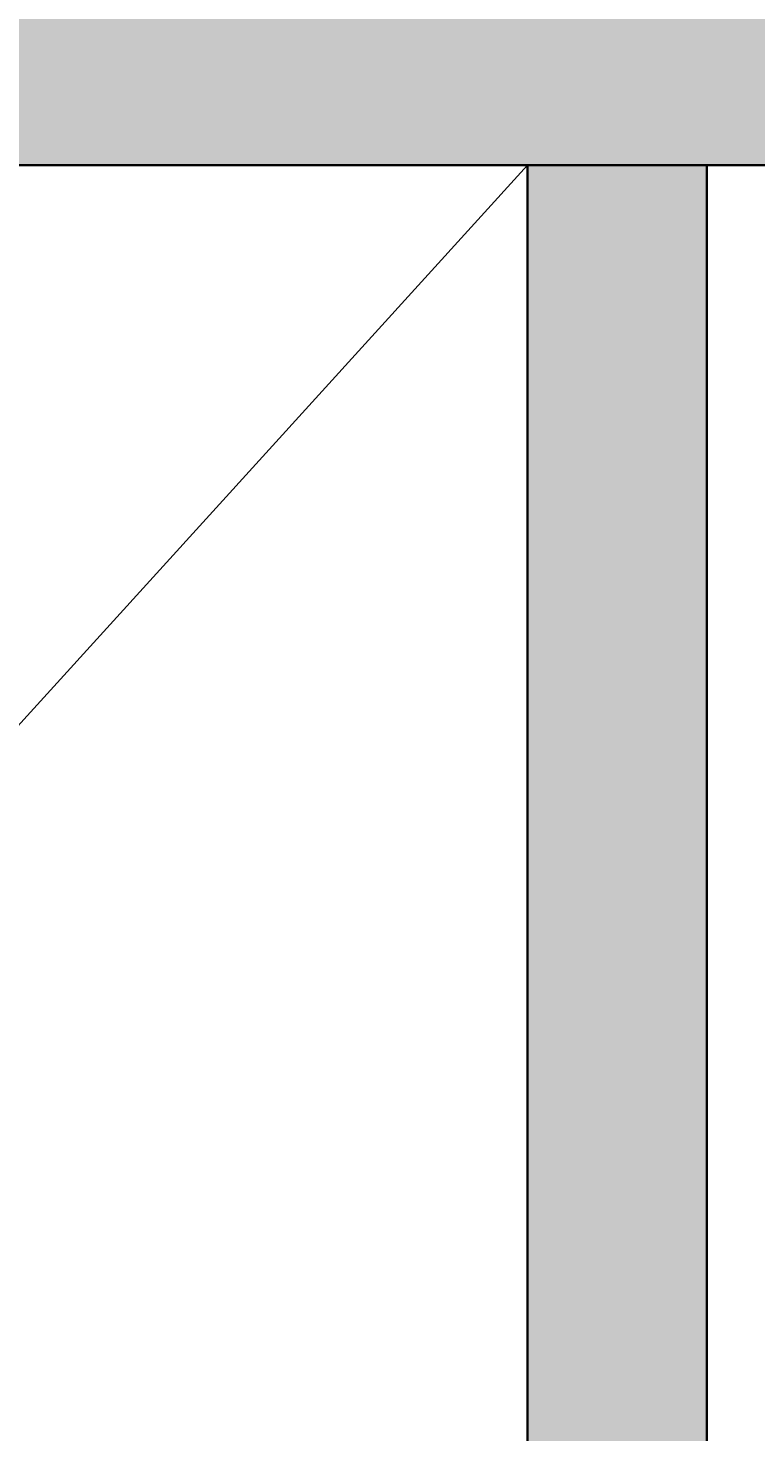
# Model space of a CAD drawing. Units: inches. Extents: x 1998 to 2588, y 1139 to 1977.
# Tile 38 of 134: x 2275 to 2293, y 1557 to 1592. Entities that reach past the tile are written whole.
import ezdxf

# ---------------------------------------------------------------- set-up
doc = ezdxf.new("R2010")
doc.units = ezdxf.units.IN
for name, color, linetype, lineweight in [('A-ANNO-DIMS', 2, 'Continuous', 18), ('A-FLOR-OPEN', 8, 'Continuous', 18), ('A-WALL-PATT', 252, 'Continuous', 13), ('WALL', 200, 'Continuous', 35)]:
    doc.layers.add(name, color=color, linetype=linetype, lineweight=lineweight)
doc.styles.get("Standard").update_dxf_attribs({"font": 'arial.ttf'})
doc.dimstyles.get("Standard").update_dxf_attribs({"dimtxt": 0.18, "dimasz": 0.18, "dimexe": 0.18, "dimexo": 0.0625, "dimgap": 0.09, "dimtad": 0, "dimtih": 1, "dimtoh": 1, "dimdec": 4, "dimzin": 0, "dimdsep": 46, "dimtxsty": 'Standard', "dimcen": 0.09, "dimadec": 0, "dimazin": 0, "dimtfac": 1, "dimtdec": 4, "dimtofl": 0, "dimtmove": 0, "dimatfit": 3, "dimfxl": 1, "dimtolj": 1, "dimtzin": 0, "dimarcsym": 0})

# ---------------------------------------------------------------- blocks, each defined once
blk = doc.blocks.new('*D34')
at = {"layer": 'A-ANNO-DIMS', "color": 0, "lineweight": -2, "transparency": 16777216}
for p, q in [((2407.91, 1594.732), (1997.843, 1594.732)), ((1998.023, 1594.552), (1998.023, 1558.913)), ((1998.023, 1522.912), (1998.023, 1558.552)), ((2407.91, 1522.732), (1997.843, 1522.732))]:
    blk.add_line(p, q, dxfattribs=at)
at = {"layer": 'A-ANNO-DIMS', "color": 0, "transparency": 16777216}
for points in [[(1997.993, 1594.552), (1998.053, 1594.552), (1998.023, 1594.732)], [(1997.993, 1522.912), (1998.053, 1522.912), (1998.023, 1522.732)]]:
    blk.add_solid(points, dxfattribs=at)
at = {"layer": 'Defpoints', "color": 0, "transparency": 16777216}
for p in [(1998.023, 1594.732), (2407.973, 1594.732), (2407.973, 1522.732)]:
    blk.add_point(p, dxfattribs=at)
at = {"layer": 'A-ANNO-DIMS', "color": 0, "transparency": 16777216, "insert": (1998.023, 1558.732), "char_height": 0.18, "attachment_point": 5}
blk.add_mtext('\\A1;72', dxfattribs=at)
blk = doc.blocks.new('*D41')
at = {"layer": 'A-ANNO-DIMS', "color": 0, "lineweight": -2, "transparency": 16777216}
for p, q in [((2227.473, 1588.67), (2227.473, 1138.602)), ((2287.473, 1588.67), (2287.473, 1138.602)), ((2227.653, 1138.782), (2257.254, 1138.782)), ((2287.293, 1138.782), (2257.692, 1138.782))]:
    blk.add_line(p, q, dxfattribs=at)
at = {"layer": 'A-ANNO-DIMS', "color": 0, "transparency": 16777216}
for points in [[(2227.653, 1138.812), (2227.653, 1138.752), (2227.473, 1138.782)], [(2287.293, 1138.812), (2287.293, 1138.752), (2287.473, 1138.782)]]:
    blk.add_solid(points, dxfattribs=at)
at = {"layer": 'Defpoints', "color": 0, "transparency": 16777216}
for p in [(2227.473, 1588.732), (2287.473, 1588.732), (2287.473, 1138.782)]:
    blk.add_point(p, dxfattribs=at)
at = {"layer": 'A-ANNO-DIMS', "color": 0, "transparency": 16777216, "insert": (2257.473, 1138.782), "char_height": 0.18, "attachment_point": 5}
blk.add_mtext('\\A1;60', dxfattribs=at)
blk = doc.blocks.new('*D42')
at = {"layer": 'A-ANNO-DIMS', "color": 0, "lineweight": -2, "transparency": 16777216}
for p, q in [((2287.535, 1588.732), (2588.309, 1588.732)), ((2588.129, 1588.552), (2588.129, 1555.914)), ((2588.129, 1522.912), (2588.129, 1555.55)), ((2287.535, 1522.732), (2588.309, 1522.732))]:
    blk.add_line(p, q, dxfattribs=at)
at = {"layer": 'A-ANNO-DIMS', "color": 0, "transparency": 16777216}
for points in [[(2588.099, 1588.552), (2588.159, 1588.552), (2588.129, 1588.732)], [(2588.099, 1522.912), (2588.159, 1522.912), (2588.129, 1522.732)]]:
    blk.add_solid(points, dxfattribs=at)
at = {"layer": 'Defpoints', "color": 0, "transparency": 16777216}
for p in [(2287.473, 1588.732), (2588.129, 1588.732), (2287.473, 1522.732)]:
    blk.add_point(p, dxfattribs=at)
at = {"layer": 'A-ANNO-DIMS', "color": 0, "transparency": 16777216, "insert": (2588.129, 1555.732), "char_height": 0.18, "attachment_point": 5}
blk.add_mtext('\\A1;66', dxfattribs=at)

msp = doc.modelspace()

# ---------------------------------------------------------------- hatches: boundary and pattern name
at = {"layer": 'A-WALL-PATT'}
h = msp.add_hatch(color=256, dxfattribs=at)
h.dxf.hatch_style = 1
h.paths.add_polyline_path([(2222.9729, 1888.7324), (2099.4125, 1888.7324), (2099.4125, 1879.7324), (2222.9729, 1879.7324)])
h.paths.add_polyline_path([(2096.9729, 1868.3278), (2087.9729, 1868.3278), (2087.9729, 1775.637), (2096.9729, 1775.637)])
h.paths.add_polyline_path([(2227.4729, 1868.3278), (2222.9729, 1868.3278), (2222.9729, 1774.3318), (2227.4729, 1774.3318)])
h.paths.add_polyline_path([(2188.3019, 1759.7324), (2138.6074, 1759.7324), (2099.4125, 1759.7324), (2099.4125, 1755.2324), (2176.9729, 1755.2324), (2188.3019, 1755.2324)])
h.paths.add_polyline_path([(2087.9729, 1759.7324), (2059.4729, 1759.7324), (2059.4729, 1702.7324), (2087.9729, 1702.7324), (2087.9729, 1707.2324), (2063.9729, 1707.2324), (2063.9729, 1755.2324), (2087.9729, 1755.2324)])
h.paths.add_polyline_path([(2096.9729, 1755.2324), (2087.9729, 1755.2324), (2087.9729, 1707.2324), (2096.9729, 1707.2324)])
h.paths.add_polyline_path([(2187.0461, 1707.2324), (2105.9729, 1707.2324), (2096.9729, 1707.2324), (2087.9729, 1707.2324), (2087.9729, 1702.7324), (2105.9729, 1702.7324), (2114.9729, 1702.7324), (2187.0461, 1702.7324)])
h.paths.add_polyline_path([(2181.4729, 1719.2028), (2176.9729, 1719.2028), (2176.9729, 1707.2324), (2181.4729, 1707.2324)])
h.paths.add_polyline_path([(2216.0332, 1588.7324), (2114.9729, 1588.7324), (2105.9729, 1588.7324), (2105.9729, 1584.2324), (2216.0332, 1584.2324)])
h.paths.add_polyline_path([(2077.691, 1588.7324), (2061.4729, 1588.7324), (2061.4729, 1584.2324), (2077.691, 1584.2324)])
h.paths.add_polyline_path([(2105.9729, 1588.7324), (2098.0956, 1588.7324), (2098.0956, 1584.2324), (2105.9729, 1584.2324)])
h.paths.add_polyline_path([(2114.9729, 1596.2642), (2110.1012, 1596.2642), (2105.9729, 1596.2642), (2105.9729, 1588.7324), (2114.9729, 1588.7324)])
h.paths.add_polyline_path([(2114.9729, 1584.2324), (2105.9729, 1584.2324), (2105.9729, 1580.249), (2110.1012, 1580.249), (2114.9729, 1580.249)])
h.paths.add_polyline_path([(2114.9729, 1547.7716), (2110.1012, 1547.7716, -0.0318759), (2105.9729, 1548.035), (2105.9729, 1470.2324), (2108.3775, 1470.2324), (2108.3775, 1465.7324), (2186.2943, 1465.7324), (2186.2943, 1470.2324), (2114.9729, 1470.2324)])
h.paths.add_polyline_path([(2227.4729, 1584.2324), (2222.9729, 1584.2324), (2222.9729, 1486.137), (2227.4729, 1486.137)])
h.paths.add_polyline_path([(2295.4138, 1593.2324), (2227.4729, 1593.2324), (2227.4729, 1588.7324), (2295.4138, 1588.7324), (2295.4138, 1591.8729)])
h.paths.add_polyline_path([(2345.9729, 1627.1165), (2341.4729, 1627.1165), (2341.4729, 1593.2324), (2337.2869, 1593.2324), (2337.2869, 1591.8729), (2337.2869, 1588.7324), (2345.9729, 1588.7324)])
h.paths.add_polyline_path([(2291.9729, 1588.7324), (2287.4729, 1588.7324), (2287.4729, 1522.7324), (2291.9729, 1522.7324)])
h.paths.add_polyline_path([(2291.9729, 1522.7324), (2287.4729, 1522.7324), (2227.4729, 1522.7324), (2227.4729, 1518.2324), (2291.9729, 1518.2324)])
h.paths.add_polyline_path([(2295.7347, 1519.5919), (2295.7347, 1522.7324), (2291.9729, 1522.7324), (2291.9729, 1518.2324), (2295.7347, 1518.2324)])
h.paths.add_polyline_path([(2345.9729, 1522.7324), (2337.6078, 1522.7324), (2337.6078, 1519.5919), (2337.6078, 1518.2324), (2341.4729, 1518.2324), (2341.4729, 1488.5616), (2345.9729, 1488.5616)])
h.paths.add_polyline_path([(2345.9729, 1468.1569), (2341.4729, 1468.1569), (2341.4729, 1374.2324), (2227.4729, 1374.2324), (2227.4729, 1369.7324), (2345.9729, 1369.7324)])
h.paths.add_polyline_path([(2345.9729, 1369.7324), (2341.4729, 1369.7324), (2341.4729, 1362.2324), (2345.9729, 1362.2324)])
h.paths.add_polyline_path([(2345.9729, 1317.7324), (2345.9729, 1322.2324), (2341.4729, 1322.2324), (2341.4729, 1285.137), (2345.9729, 1285.137)], flags=17)
h.paths.add_polyline_path([(2356.2096, 1322.2324), (2345.9729, 1322.2324), (2345.9729, 1317.7324), (2356.2096, 1317.7324), (2356.2096, 1319.3088)], flags=17)
h.paths.add_polyline_path([(2393.9729, 1322.2324), (2375.6999, 1322.2324), (2375.6999, 1319.3088, -0.0202458), (2375.636, 1317.7324), (2393.9729, 1317.7324)], flags=17)
h.paths.add_polyline_path([(2398.4729, 1322.2324), (2393.9729, 1322.2324), (2393.9729, 1317.7324), (2393.9729, 1237.7324), (2345.9729, 1237.7324), (2345.9729, 1264.7324), (2341.4729, 1264.7324), (2341.4729, 1228.7324), (2393.9729, 1228.7324), (2482.7412, 1228.7324), (2482.7412, 1237.7324), (2398.4729, 1237.7324), (2398.4729, 1297.1029)])
h.paths.add_polyline_path([(2398.4729, 1362.2324), (2393.9729, 1362.2324), (2393.9729, 1357.7324), (2398.4729, 1357.7324)])
h.paths.add_polyline_path([(2345.9729, 1329.7549), (2341.4729, 1329.7549), (2341.4729, 1322.2324), (2345.9729, 1322.2324)])

# ---------------------------------------------------------------- linework, layer by layer
at = {"layer": 'A-FLOR-OPEN'}
msp.add_line((2227.4729, 1522.7324), (2287.4729, 1588.7324), dxfattribs=at)
at = {"layer": 'WALL'}
for p, q in [((2295.4138, 1588.7324), (2227.4729, 1588.7324)), ((2287.4729, 1522.7324), (2287.4729, 1588.7324)), ((2291.9729, 1518.2324), (2291.9729, 1588.7324))]:
    msp.add_line(p, q, dxfattribs=at)

# ---------------------------------------------------------------- dimensions: what is measured, and where the dimension line sits
at = {"layer": 'A-ANNO-DIMS'}
for base, p1, p2, picture, middle in [((1998.0229, 1594.7324), (2407.9729, 1522.7324), (2407.9729, 1594.7324), '*D34', (1998.0229, 1558.7324)), ((2588.1286, 1588.7324), (2287.4729, 1522.7324), (2287.4729, 1588.7324), '*D42', (2588.1286, 1555.7324))]:
    dim = msp.add_linear_dim(base=base, p1=p1, p2=p2, angle=90, dimstyle='Standard', override={"dimdec": 0, "dimlfac": 1, "dimrnd": 0, "dimzin": 0, "dimdsep": 46, "dimlunit": 2}, dxfattribs=at)
    dim.commit()
    dim.dimension.update_dxf_attribs({"geometry": picture, "text_midpoint": middle})
dim = msp.add_linear_dim(base=(2287.4729, 1138.7824), p1=(2227.4729, 1588.7324), p2=(2287.4729, 1588.7324), dimstyle='Standard', override={"dimdec": 0, "dimlfac": 1, "dimrnd": 0, "dimzin": 0, "dimdsep": 46, "dimlunit": 2}, dxfattribs=at)
dim.commit()
dim.dimension.update_dxf_attribs({"geometry": '*D41', "text_midpoint": (2257.4729, 1138.7824)})

doc.saveas('drawing.dxf')
